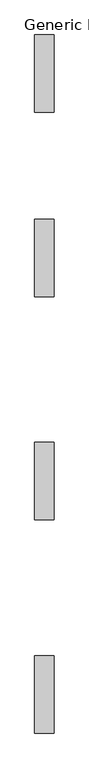
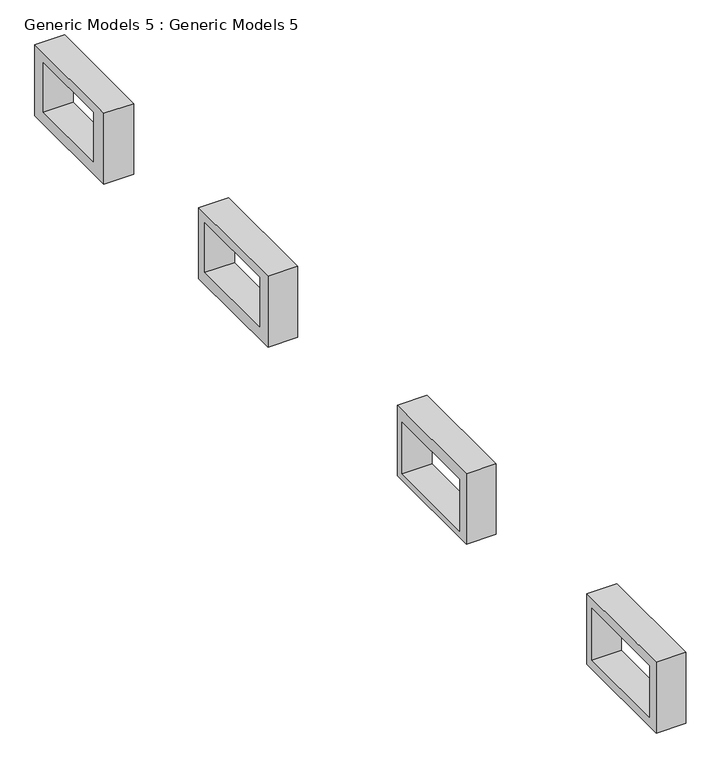
"""IFC4 building model written with IfcOpenShell, lengths in millimetres: proxy geometry, Generic Models 5 : Generic Models 5."""

from ifc_helpers import new_model, si_unit, frame, origin, place, context, project, spatial, polyline, outline, extrude, source, transform, mapped, element, save


def generic_models_5_generic_models_5_c5eedb73(model_context):
    return source(origin(), model_context, "Body", "SweptSolid", [
        extrude(outline(polyline([(-3477.9860806, 1109.6193499), (-3477.9860806, 347.6193499), (-4697.1860806, 347.6193499), (-4697.1860806, 1109.6193499), (-3477.9860806, 1109.6193499)]), holes=[polyline([(-3559.4540407, 442.6024779), (-3559.4540407, 1001.4024779), (-4575.4540407, 1001.4024779), (-4575.4540407, 442.6024779), (-3559.4540407, 442.6024779)])]), frame((3554.7910386, 0.0, 0.0), z_axis=(1.0, 0.0, 0.0), x_axis=(0.0, 1.0, 0.0)), (0.0, 0.0, 1.0), 304.8),
        extrude(outline(polyline([(-125.1860806, 1109.6193499), (-125.1860806, 347.6193499), (-1344.3860806, 347.6193499), (-1344.3860806, 1109.6193499), (-125.1860806, 1109.6193499)]), holes=[polyline([(-207.4231106, 417.7143445), (-207.4231106, 976.5143445), (-1223.4231106, 976.5143445), (-1223.4231106, 417.7143445), (-207.4231106, 417.7143445)])]), frame((3554.7910386, 0.0, 0.0), z_axis=(1.0, 0.0, 0.0), x_axis=(0.0, 1.0, 0.0)), (0.0, 0.0, 1.0), 304.8),
        extrude(outline(polyline([(3380.0139194, 1109.6193499), (3380.0139194, 347.6193499), (2160.8139194, 347.6193499), (2160.8139194, 1109.6193499), (3380.0139194, 1109.6193499)]), holes=[polyline([(3276.0039871, 475.6061876), (3276.0039871, 1009.0061876), (2310.8039871, 1009.0061876), (2310.8039871, 475.6061876), (3276.0039871, 475.6061876)])]), frame((3554.7910386, 0.0, 0.0), z_axis=(1.0, 0.0, 0.0), x_axis=(0.0, 1.0, 0.0)), (0.0, 0.0, 1.0), 304.8),
        extrude(outline(polyline([(6275.6139194, 1109.6193499), (6275.6139194, 347.6193499), (5056.4139194, 347.6193499), (5056.4139194, 1109.6193499), (6275.6139194, 1109.6193499)]), holes=[polyline([(6125.7329839, 475.6061876), (6125.7329839, 1009.0061876), (5246.6906096, 1009.0061876), (5246.6906096, 475.6061876), (6125.7329839, 475.6061876)])]), frame((3554.7910386, 0.0, 0.0), z_axis=(1.0, 0.0, 0.0), x_axis=(0.0, 1.0, 0.0)), (0.0, 0.0, 1.0), 304.8),
    ])


if __name__ == "__main__":
    model = new_model("IFC4")
    model_context = context("Model", 3, world=origin())
    ifc_project = project(units=[si_unit("LENGTHUNIT", "METRE", prefix="MILLI")], contexts=[model_context])
    site = spatial("IfcSite", under=ifc_project)
    building = spatial("IfcBuilding", under=site)
    placement = place(None, origin())
    generic_models_5_generic_models_5_shape = generic_models_5_generic_models_5_c5eedb73(model_context)
    element("IfcBuildingElementProxy", 1, Name="Generic Models 5 : Generic Models 5", ObjectType="Generic Models 5 : Generic Models 5", at=placement, inside=building, context=model_context, shape_type="MappedRepresentation", body=[
        mapped(generic_models_5_generic_models_5_shape, transform((0.0, 0.0, 0.0), x_axis=(1.0, 0.0, 0.0), y_axis=(0.0, 1.0, 0.0), z_axis=(0.0, 0.0, 1.0))),
    ])
    save(model, "model.ifc")

# Revit data of these elements
# Element 1 (IfcBuildingElementProxy, "Generic Models 5 : Generic Models 5")
#   Materials on its faces: "Parking Stripe"
# Materials
#   "Parking Stripe": class "Paint", colour RGB 250 250 91, transparency 0, Cost = 0
